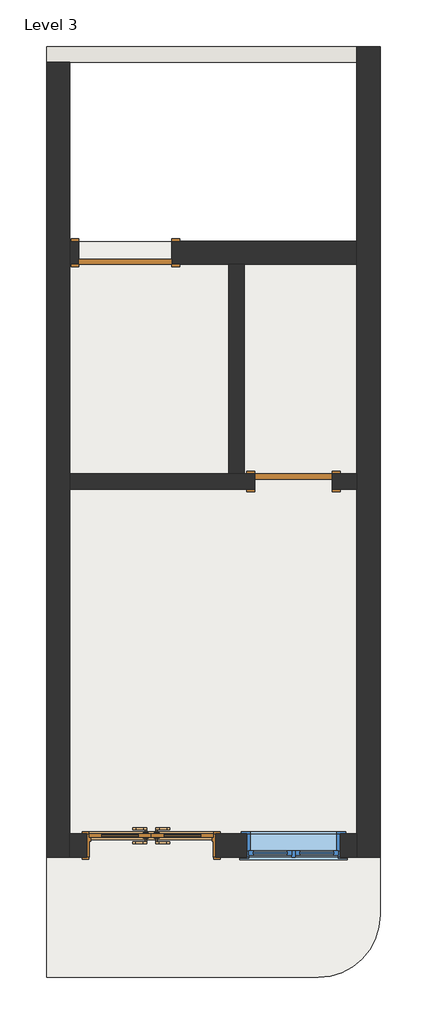
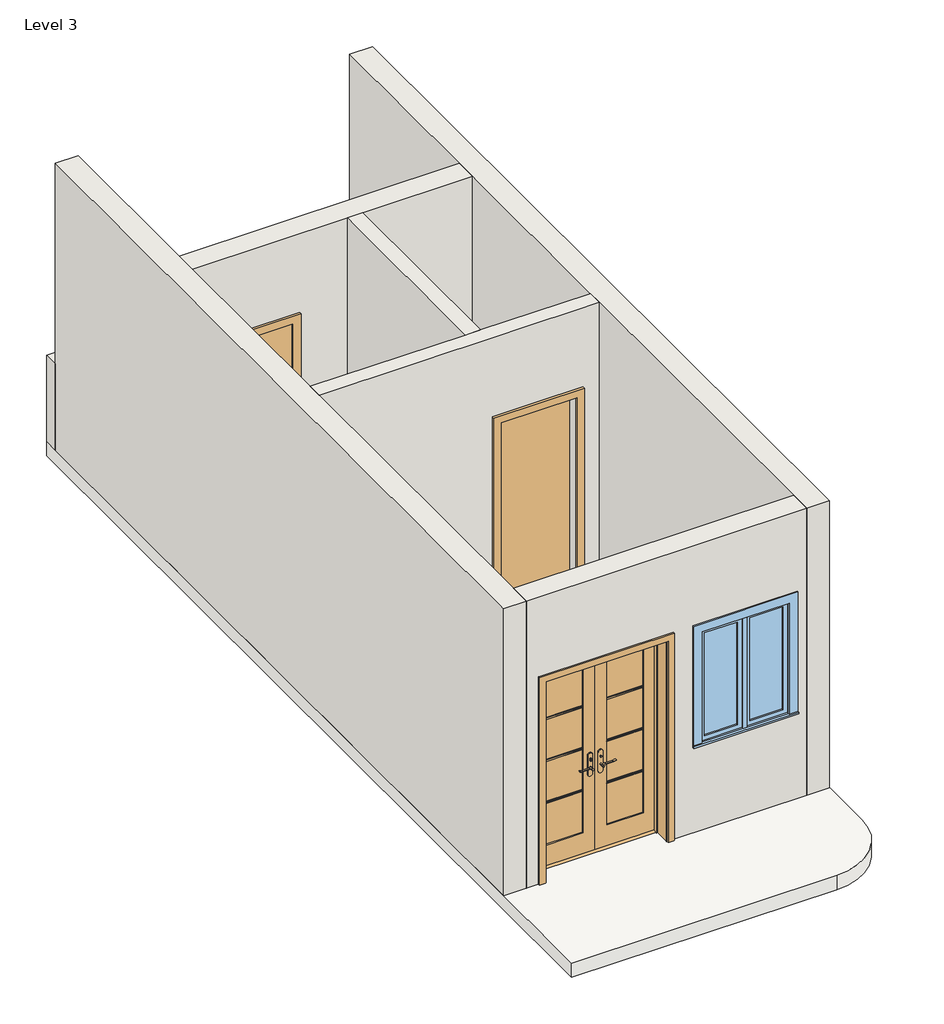
# One storey, incomplete: 7 walls, 3 doors, 1 slab, 1 window.
"""IFC4 building model written with IfcOpenShell, lengths in millimetres."""

from ifc_helpers import new_model, si_unit, point, frame, frame_2d, origin, place, context, project, spatial, polyline, circle_curve, trimmed, segment, composite_curve, outline, extrude, faceted_brep, transform, mapped, element, save
from components import door_4500b467, single_flush_2_5_e2b13fe9, door_0ca8825f, window_419b5846

model = new_model("IFC4")

# Units and contexts
model_context = context("Model", 3, world=origin())
ifc_project = project(units=[si_unit("LENGTHUNIT", "METRE", prefix="MILLI")], contexts=[model_context])

# Site, building, storey
site = spatial("IfcSite", under=ifc_project)
building = spatial("IfcBuilding", under=site)
storey = spatial("IfcBuildingStorey", under=building, Name="Level 3", Elevation=6400.8)

# Doors
placement = place(None, origin())
door_shape = door_4500b467(model_context)
element("IfcDoor", 1, ObjectType="Door-Exterior-Double-Full Glass-Wood_Clad : 48\" x 84\"", at=placement, inside=storey, context=model_context, shape_type="MappedRepresentation", body=[
    mapped(door_shape, transform((-5892.5189081, -995.3847011, 6400.8), x_axis=(1.0, 0.0, 0.0), y_axis=(0.0, 1.0, 0.0), z_axis=(0.0, 0.0, 1.0))),
])
single_flush_2_5_shape = single_flush_2_5_e2b13fe9(model_context)
element("IfcDoor", 2, ObjectType="Single-Flush : 2.5'", at=placement, inside=storey, context=model_context, shape_type="MappedRepresentation", body=[
    mapped(single_flush_2_5_shape, transform((-4495.5189081, 2576.4902989, 6400.8), x_axis=(-1.0, 0.0, 0.0), y_axis=(0.0, -1.0, 0.0), z_axis=(0.0, 0.0, 1.0))),
])
door_2_shape = door_0ca8825f(model_context)
element("IfcDoor", 3, ObjectType="Single-Flush : 36\" x 84\"", at=placement, inside=storey, context=model_context, shape_type="MappedRepresentation", body=[
    mapped(door_2_shape, transform((-6146.5189081, 4824.3902989, 6400.8), x_axis=(-1.0, 0.0, 0.0), y_axis=(0.0, -1.0, 0.0), z_axis=(0.0, 0.0, 1.0))),
])

# Slab
element("IfcSlab", 4, ObjectType="6\"", at=placement, inside=storey, context=model_context, shape_type="SweptSolid", body=[
    extrude(outline(composite_curve([segment(polyline([(-3644.6189081, 6850.0402989), (-3644.6189081, -1684.3597011)]), True, "CONTINUOUS"), segment(trimmed(circle_curve(frame_2d((-4254.2189081, -1684.3597011)), 609.6), [point((-3644.6189081, -1684.3597011))], [point((-4254.2189081, -2293.9597011))], False, "CARTESIAN"), True, "CONTINUOUS"), segment(polyline([(-4254.2189081, -2293.9597011), (-6921.2189081, -2293.9597011), (-6921.2189081, 6850.0402989), (-3644.6189081, 6850.0402989)]), True, "CONTINUOUS")], self_intersect=False), holes=[polyline([(-3873.2189081, 4938.1100028), (-3873.2189081, 6697.6402989), (-6692.6189081, 6697.6402989), (-6692.6189081, 4938.1100028), (-3873.2189081, 4938.1100028)])]), frame((0.0, 0.0, 6248.4), z_axis=(0.0, 0.0, 1.0), x_axis=(1.0, 0.0, 0.0)), (0.0, 0.0, 1.0), 152.4),
])

# Walls
element("IfcWall", 5, ObjectType="6\"", at=placement, inside=storey, context=model_context, shape_type="Brep", body=[
    faceted_brep([(-6921.2189081, 6697.6402989, 6400.8), (-6692.6189081, 6697.6402989, 6400.8), (-3873.2189081, 6697.6402989, 6400.8), (-3873.2189081, 6697.6402989, 7315.2), (-6921.2189081, 6697.6402989, 7315.2), (-6921.2189081, 6850.0402989, 6400.8), (-6921.2189081, 6850.0402989, 7315.2), (-3873.2189081, 6850.0402989, 7315.2), (-3873.2189081, 6850.0402989, 6400.8)], [[[0, 1, 2, 3, 4]], [[5, 6, 7, 8]], [[2, 1, 0, 5, 8]], [[4, 3, 7, 6]], [[0, 4, 6, 5]], [[3, 2, 8, 7]]]),
])
element("IfcWall", 6, ObjectType="6\"", at=placement, inside=storey, context=model_context, shape_type="Brep", body=[
    faceted_brep([(-4876.5189081, 2652.6902989, 8534.4), (-4876.5189081, 2652.6902989, 6400.8), (-4978.1189081, 2652.6902989, 6400.8), (-5130.5189081, 2652.6902989, 6400.8), (-6692.6189081, 2652.6902989, 6400.8), (-6692.6189081, 2652.6902989, 9448.8), (-5130.5189081, 2652.6902989, 9448.8), (-4978.1189081, 2652.6902989, 9448.8), (-3873.2189081, 2652.6902989, 9448.8), (-3873.2189081, 2652.6902989, 6400.8), (-4114.5189081, 2652.6902989, 6400.8), (-4114.5189081, 2652.6902989, 8534.4), (-6692.6189081, 2500.2902989, 6400.8), (-4876.5189081, 2500.2902989, 6400.8), (-4876.5189081, 2500.2902989, 8534.4), (-4114.5189081, 2500.2902989, 8534.4), (-4114.5189081, 2500.2902989, 6400.8), (-3873.2189081, 2500.2902989, 6400.8), (-3873.2189081, 2500.2902989, 9448.8), (-6692.6189081, 2500.2902989, 9448.8)], [[[0, 1, 2, 3, 4, 5, 6, 7, 8, 9, 10, 11]], [[12, 13, 14, 15, 16, 17, 18, 19]], [[10, 9, 17, 16]], [[4, 3, 2, 1, 13, 12]], [[8, 7, 6, 5, 19, 18]], [[5, 4, 12, 19]], [[9, 8, 18, 17]], [[14, 13, 1, 0]], [[15, 14, 0, 11]], [[16, 15, 11, 10]]]),
])
element("IfcWall", 7, ObjectType="6\"", at=placement, inside=storey, context=model_context, shape_type="SweptSolid", body=[
    extrude(outline(polyline([(-4978.1189081, 4710.0902989), (-4978.1189081, 2652.6902989), (-5130.5189081, 2652.6902989), (-5130.5189081, 4710.0902989), (-4978.1189081, 4710.0902989)])), frame((0.0, 0.0, 6400.8), z_axis=(0.0, 0.0, 1.0), x_axis=(1.0, 0.0, 0.0)), (0.0, 0.0, 1.0), 3048.0),
])
element("IfcWall", 8, ObjectType="9\"", at=placement, inside=storey, context=model_context, shape_type="Brep", body=[
    faceted_brep([(-3873.2189081, 6850.0402989, 6400.8), (-3873.2189081, 6697.6402989, 6400.8), (-3873.2189081, 4938.6902989, 6400.8), (-3873.2189081, 4710.0902989, 6400.8), (-3873.2189081, 2652.6902989, 6400.8), (-3873.2189081, 2500.2902989, 6400.8), (-3873.2189081, -884.2597011, 6400.8), (-3873.2189081, -1112.8597011, 6400.8), (-3873.2189081, -1112.8597011, 9448.8), (-3873.2189081, -884.2597011, 9448.8), (-3873.2189081, 2500.2902989, 9448.8), (-3873.2189081, 2652.6902989, 9448.8), (-3873.2189081, 4710.0902989, 9448.8), (-3873.2189081, 4938.6902989, 9448.8), (-3873.2189081, 6850.0402989, 9448.8), (-3873.2189081, 6850.0402989, 7315.2), (-3644.6189081, 6850.0402989, 6400.8), (-3644.6189081, 6850.0402989, 9448.8), (-3644.6189081, -1112.8597011, 9448.8), (-3644.6189081, -1112.8597011, 6400.8)], [[[0, 1, 2, 3, 4, 5, 6, 7, 8, 9, 10, 11, 12, 13, 14, 15]], [[16, 17, 18, 19]], [[7, 6, 5, 4, 3, 2, 1, 0, 16, 19]], [[14, 13, 12, 11, 10, 9, 8, 18, 17]], [[0, 15, 14, 17, 16]], [[8, 7, 19, 18]]]),
])
element("IfcWall", 9, ObjectType="9\"", at=placement, inside=storey, context=model_context, shape_type="Brep", body=[
    faceted_brep([(-6603.7189081, 4938.6902989, 8534.4), (-6603.7189081, 4938.6902989, 6400.8), (-6692.6189081, 4938.6902989, 6400.8), (-6692.6189081, 4938.6902989, 9448.8), (-3873.2189081, 4938.6902989, 9448.8), (-3873.2189081, 4938.6902989, 6400.8), (-5689.3189081, 4938.6902989, 6400.8), (-5689.3189081, 4938.6902989, 8534.4), (-6692.6189081, 4710.0902989, 6400.8), (-6603.7189081, 4710.0902989, 6400.8), (-6603.7189081, 4710.0902989, 8534.4), (-5689.3189081, 4710.0902989, 8534.4), (-5689.3189081, 4710.0902989, 6400.8), (-5130.5189081, 4710.0902989, 6400.8), (-4978.1189081, 4710.0902989, 6400.8), (-3873.2189081, 4710.0902989, 6400.8), (-3873.2189081, 4710.0902989, 9448.8), (-4978.1189081, 4710.0902989, 9448.8), (-5130.5189081, 4710.0902989, 9448.8), (-6692.6189081, 4710.0902989, 9448.8)], [[[0, 1, 2, 3, 4, 5, 6, 7]], [[8, 9, 10, 11, 12, 13, 14, 15, 16, 17, 18, 19]], [[6, 5, 15, 14, 13, 12]], [[2, 1, 9, 8]], [[4, 3, 19, 18, 17, 16]], [[3, 2, 8, 19]], [[5, 4, 16, 15]], [[10, 9, 1, 0]], [[11, 10, 0, 7]], [[12, 11, 7, 6]]]),
])
element("IfcWall", 10, ObjectType="9\"", at=placement, inside=storey, context=model_context, shape_type="SweptSolid", body=[
    extrude(outline(polyline([(9448.8, -3873.2189081), (9448.8, -6692.6189081), (6400.8, -6692.6189081), (6400.8, -6527.5189081), (8559.8, -6527.5189081), (8559.8, -5257.5189081), (6400.8, -5257.5189081), (6400.8, -3873.2189081), (9448.8, -3873.2189081)]), holes=[polyline([(8534.4, -4952.7189081), (8534.4, -4038.3189081), (7315.2, -4038.3189081), (7315.2, -4952.7189081), (8534.4, -4952.7189081)])]), frame((0.0, -1112.8597011, 0.0), z_axis=(0.0, 1.0, 0.0), x_axis=(0.0, 0.0, 1.0)), (0.0, 0.0, 1.0), 228.6),
])
element("IfcWall", 11, ObjectType="9\"", at=placement, inside=storey, context=model_context, shape_type="Brep", body=[
    faceted_brep([(-6692.6189081, -1112.8597011, 6400.8), (-6692.6189081, -884.2597011, 6400.8), (-6692.6189081, 2500.2902989, 6400.8), (-6692.6189081, 2652.6902989, 6400.8), (-6692.6189081, 4710.0902989, 6400.8), (-6692.6189081, 4938.6902989, 6400.8), (-6692.6189081, 6697.6402989, 6400.8), (-6692.6189081, 6697.6402989, 9448.8), (-6692.6189081, 4938.6902989, 9448.8), (-6692.6189081, 4710.0902989, 9448.8), (-6692.6189081, 2652.6902989, 9448.8), (-6692.6189081, 2500.2902989, 9448.8), (-6692.6189081, -884.2597011, 9448.8), (-6692.6189081, -1112.8597011, 9448.8), (-6921.2189081, -1112.8597011, 6400.8), (-6921.2189081, -1112.8597011, 9448.8), (-6921.2189081, 6697.6402989, 9448.8), (-6921.2189081, 6697.6402989, 7315.2), (-6921.2189081, 6697.6402989, 6400.8)], [[[0, 1, 2, 3, 4, 5, 6, 7, 8, 9, 10, 11, 12, 13]], [[14, 15, 16, 17, 18]], [[6, 5, 4, 3, 2, 1, 0, 14, 18]], [[13, 12, 11, 10, 9, 8, 7, 16, 15]], [[7, 6, 18, 17, 16]], [[0, 13, 15, 14]]]),
])

# Window
window_shape = window_419b5846(model_context)
element("IfcWindow", 12, ObjectType="Casement Dbl with Trim : 36\" x 48\"", at=placement, inside=storey, context=model_context, shape_type="MappedRepresentation", body=[
    mapped(window_shape, transform((-4495.5189081, -979.5097011, 6400.8), x_axis=(-1.0, 0.0, 0.0), y_axis=(0.0, -1.0, 0.0), z_axis=(0.0, 0.0, 1.0))),
])

save(model, "model.ifc")

# Revit data of these elements
# Type "Door-Exterior-Double-Full Glass-Wood_Clad : 48\" x 84\""
#   Type Mark = "9"
#   Assembly Code = "B2030100"
#   Analytic Construction = "French door, wood frame with double glass"
#   Top Rail = 0' - 4 11/16"
#   Threshold Offset [instance default] = 0' - 0 1/2"
#   Thickness = 0' - 1 3/8"
#   Thermal Resistance (R) = 1.9158 (h·ft²·°F)/BTU
#   Swing Angle [instance default] = 90.00°
#   Stiles = 0' - 4 3/4"
#   Rough Width = 4' - 2"
#   Rough Height = 7' - 1"
#   Panel Width = 2' - 0"
#   Door Offset [instance default] = 0' - 0"
#   Height = 7' - 0"
#   Width = 4' - 0"
#   Heat Transfer Coefficient (U) = 0.5220 BTU/(h·ft²·°F)
#   Bottom Rail = 0' - 9 1/8"
#   Exterior Trim [instance default] = yes
#   Threshold [instance default] = yes
#   Show Grill [instance default] = yes
#   Function = 1
#   Trim Material = Cherry
#   Threshold Material = Cherry
#   Panel Material = Cherry
#   Glazing = Glass
#   Frame Material = Cherry
#   Door Handle Material = Aluminum
#   Visual Light Transmittance = 0
#   Solar Heat Gain Coefficient = 0
#   Wall Closure = (empty or 0)
#   Construction Type = (empty or 0)
# Type "Single-Flush : 2.5'"
#   Type Mark = "8"
#   Construction Type Id = "MDOOR"
#   Assembly Code = "C1020"
#   Analytic Construction = "Metal"
#   Thickness = 0' - 2"
#   Heat Transfer Coefficient (U) = 0.651978 BTU/(h·ft²·°F)
#   Height = 7' - 0"
#   Trim Projection Ext = 0' - 1"
#   Trim Projection Int = 0' - 1"
#   Trim Width = 0' - 3"
#   Width = 2' - 6"
#   Define Thermal Properties by = 1
#   Door Material = Door - Panel
#   Frame Material = Door - Frame
#   Visual Light Transmittance = 0
#   Solar Heat Gain Coefficient = 0
#   Function = (empty or 0)
#   Wall Closure = (empty or 0)
# Type "Single-Flush : 36\" x 84\""
#   Type Mark = "1"
#   Construction Type Id = "MDOOR"
#   Assembly Code = "C1020"
#   Analytic Construction = "Metal"
#   Thickness = 0' - 2"
#   Heat Transfer Coefficient (U) = 0.651978 BTU/(h·ft²·°F)
#   Height = 7' - 0"
#   Trim Projection Ext = 0' - 1"
#   Trim Projection Int = 0' - 1"
#   Trim Width = 0' - 3"
#   Width = 3' - 0"
#   Define Thermal Properties by = 1
#   Door Material = Door - Panel
#   Frame Material = Door - Frame
#   Visual Light Transmittance = 0
#   Solar Heat Gain Coefficient = 0
#   Function = (empty or 0)
#   Wall Closure = (empty or 0)
# Type "6\""
#   Assembly Code = "B1010"
#   Function = 0
#   Layers, outside or top first: 0' - 6" no material (function 1)
# Type "6\""
#   Assembly Code = "B2010"
#   Layers, outside or top first: 0' - 6" no material (function 1)
# Type "9\""
#   Assembly Code = "B2010"
#   Layers, outside or top first: 0' - 9" no material (function 1)
# Type "Casement Dbl with Trim : 36\" x 48\""
#   Type Mark = "19"
#   Construction Type Id = "GSP4R"
#   Assembly Code = "B2020100"
#   Analytic Construction = "1/8 in Pilkington single glazing"
#   Visual Light Transmittance = 0.9
#   Solar Heat Gain Coefficient = 0.78
#   Heat Transfer Coefficient (U) = 0.6496 BTU/(h·ft²·°F)
#   Height = 4' - 0"
#   Default Sill Height = 3' - 0"
#   Trim Projection - Ext. = 0' - 0 1/2"
#   Trim Projection - Int. = 0' - 0 3/4"
#   Trim Width - Exterior = 0' - 3 1/2"
#   Trim Width - Interior = 0' - 3 1/2"
#   Width = 3' - 0"
#   Window Inset = 0' - 0 3/4"
#   Define Thermal Properties by = 1
#   Glass Pane Material = Glass
#   Sash Material = Sash
#   Trim Exterior Material = Trim
#   Trim Interior Material = Trim
#   Wall Closure = (empty or 0)
# Element 1 (IfcDoor, "Door-Exterior-Double-Full Glass-Wood_Clad : 48\" x 84\"")
#   Threshold Offset = 0' - 0 1/2"
#   Swing Angle = 90.00°
#   Door Offset = 0' - 0"
#   Threshold = yes
#   Show Grill = yes
#   Exterior Trim = yes
#   Phase Created = New Construction
#   Materials on its faces: "Cherry", "Aluminum", "Glass"
# Element 2 (IfcDoor, "Single-Flush : 2.5'")
#   Phase Created = New Construction
#   Materials on its faces: "Door - Frame", "Door - Panel"
# Element 3 (IfcDoor, "Single-Flush : 36\" x 84\"")
#   Phase Created = New Construction
#   Materials on its faces: "Door - Frame", "Door - Panel"
# Element 4 (IfcSlab, "6\"")
#   Height Offset From Level = 0' - 0"
#   Phase Created = New Construction
#   Materials on its faces: "Default Floor"
# Element 5 (IfcWall, "6\"")
#   Top Offset = 0' - 0"
#   Base Offset = 0' - 0"
#   Unconnected Height = 3' - 0"
#   wall height = 3' - 0"
#   Phase Created = New Construction
#   Base Constraint = Level 3
#   Materials on its faces: "Default Wall"
# Elements 6, 7 (IfcWall, "6\"")
#   Top Offset = 0' - 0"
#   Base Offset = 0' - 0"
#   Unconnected Height = 10' - 0"
#   wall height = 10' - 0"
#   Phase Created = New Construction
#   Base Constraint = Level 3
#   Materials on its faces: "Default Wall"
# Elements 8, 9, 10, 11 (IfcWall, "9\"")
#   Top Offset = 0' - 0"
#   Base Offset = 0' - 0"
#   Unconnected Height = 10' - 0"
#   wall height = 10' - 0"
#   Phase Created = New Construction
#   Base Constraint = Level 3
#   Materials on its faces: "Default Wall"
# Element 12 (IfcWindow, "Casement Dbl with Trim : 36\" x 48\"")
#   Mark = "4"
#   Phase Created = New Construction
#   Materials on its faces: "Sash", "Trim", "Glass"
# Materials
#   "Cherry": class "Wood", colour RGB 226 177 128, transparency 0, Description = "Prunus Serotina", Cost = 0
#   "Glass": class "Glass", colour RGB 0 128 192, transparency 0.75, Description = "Soda Lime Glass", Cost = 0
#   "Aluminum": class "Metal", colour RGB 247 247 247, transparency 0, Description = "Aluminum 6061", Cost = 0
#   "Door - Panel": class "Wood", colour RGB 210 159 95, transparency 0
#   "Door - Frame": colour RGB 118 70 51, transparency 0
#   "Sash": class "Wood", colour RGB 224 178 126, transparency 0
#   "Trim": class "Wood", colour RGB 224 178 126, transparency 0
#   "Default Floor": colour RGB 128 128 128, transparency 0
#   "Default Wall": colour RGB 128 128 128, transparency 0
